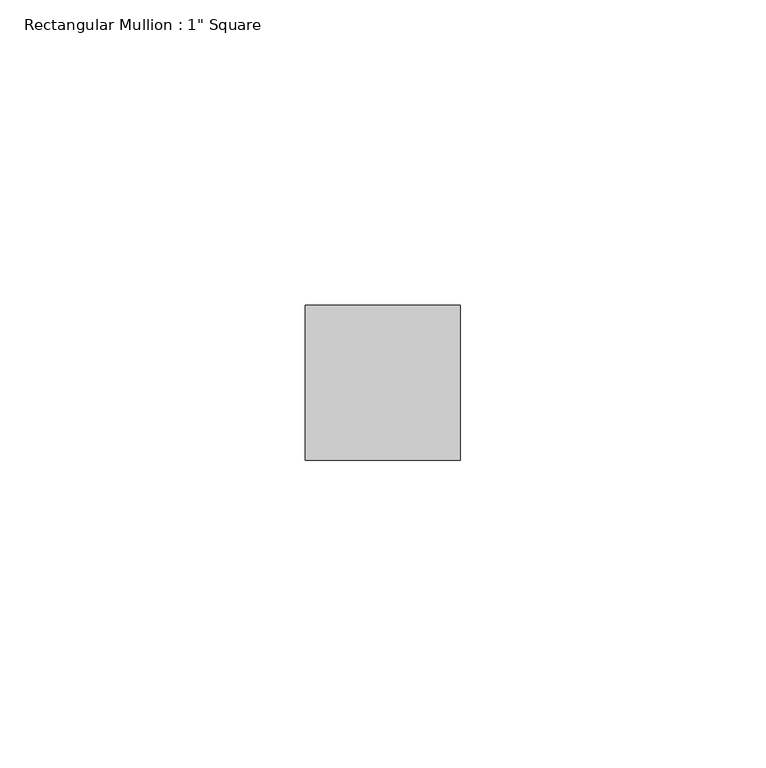
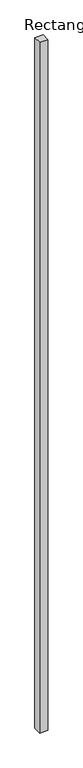
"""IFC4 building model written with IfcOpenShell, lengths in millimetres: member geometry."""

from ifc_helpers import new_model, si_unit, frame, origin, place, context, project, spatial, polyline, outline, extrude, source, transform, mapped, element, save


def member_7046656e(model_context):
    return source(origin(), model_context, "Body", "SweptSolid", [
        extrude(outline(polyline([(0.0, 12.7), (0.0, -12.7), (-25.4, -12.7), (-25.4, 12.7), (0.0, 12.7)])), frame((0.0, 0.0, -2287.5875), z_axis=(0.0, 0.0, 1.0), x_axis=(1.0, 0.0, 0.0)), (0.0, 0.0, 1.0), 2287.5875),
    ])


if __name__ == "__main__":
    model = new_model("IFC4")
    model_context = context("Model", 3, world=origin())
    ifc_project = project(units=[si_unit("LENGTHUNIT", "METRE", prefix="MILLI")], contexts=[model_context])
    site = spatial("IfcSite", under=ifc_project)
    building = spatial("IfcBuilding", under=site)
    placement = place(None, origin())
    member_shape = member_7046656e(model_context)
    element("IfcMember", 1, ObjectType="Rectangular Mullion : 1\" Square", at=placement, inside=building, context=model_context, shape_type="MappedRepresentation", body=[
        mapped(member_shape, transform((0.0, 0.0, 0.0), x_axis=(1.0, 0.0, 0.0), y_axis=(0.0, 1.0, 0.0), z_axis=(0.0, 0.0, 1.0))),
    ])
    save(model, "model.ifc")

# Revit data of these elements
# Type "Rectangular Mullion : 1\" Square"
#   built-in parameter 1007304 = 0.0833333 (stored number, unit not read)
#   built-in parameter 1007301 = 0.0416667 (stored number, unit not read)
#   built-in parameter 1007300 = 0.0416667 (stored number, unit not read)
# Element 1 (IfcMember, "Rectangular Mullion : 1\" Square")
#   Materials on its faces: "black"
# Materials
#   "black": class "Generic", colour RGB 120 120 120, transparency 0, Cost = 0
